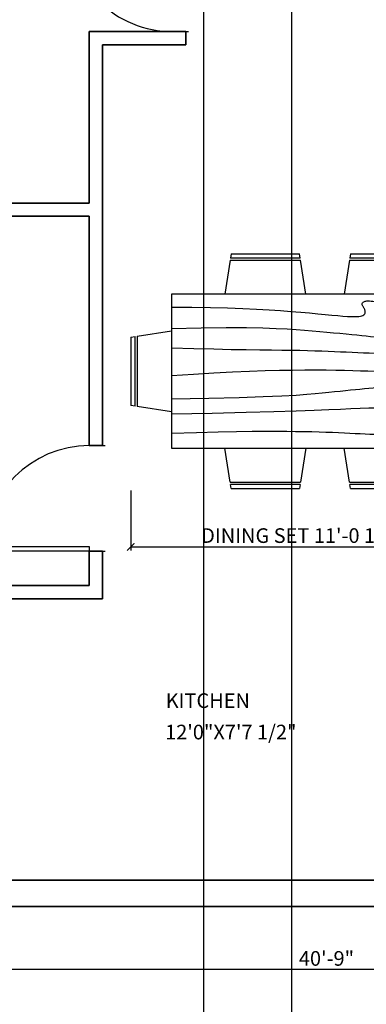
# Model space of a CAD drawing. Units: inches. Extents: x 3283068 to 3284536, y 3240756 to 3241803.
# Tile 6 of 19: x 3283479 to 3283598, y 3241165 to 3241501. Entities that reach past the tile are written whole.
import ezdxf

# ---------------------------------------------------------------- set-up
doc = ezdxf.new("R2010")
doc.units = ezdxf.units.IN
for name, color, linetype, lineweight in [('A-ANNO-DIMS', 2, 'Continuous', 18), ('A-AREA-IDEN', 7, 'Continuous', 18), ('door', 140, 'Continuous', 25), ('furniture', 40, 'Continuous', 18), ('wall', 20, 'Continuous', 35)]:
    doc.layers.add(name, color=color, linetype=linetype, lineweight=lineweight)
doc.layers.add('HATCH', color=8, linetype='Continuous')
doc.layers.add('NOI THAT', color=42, linetype='Continuous')
doc.styles.get("Standard").update_dxf_attribs({"font": 'arial.ttf'})
doc.dimstyles.new('ISO-25', dxfattribs={"dimtxt": 5, "dimasz": 2.5, "dimexe": 1.25, "dimexo": 0.625, "dimtad": 1, "dimlunit": 4, "dimtxsty": 'Standard', "dimblk": 'ARCHTICK', "dimcen": 2.5, "dimadec": 0, "dimazin": 0, "dimtfac": 1, "dimtmove": 0, "dimatfit": 3, "dimfxl": 1, "dimarcsym": 0})

# ---------------------------------------------------------------- blocks, each defined once
blk = doc.blocks.new('*U7')
for p, q in [((0, 0), (0, 6)), ((40, 0), (40, 6))]:
    blk.add_line(p, q)
blk.add_lwpolyline([(0, 0), (0, -40), (1.75, -40), (1.75, 0)], close=True)
blk.add_arc((0, 0), 40, 270, 0)
blk = doc.blocks.new('*U5')
for p, q in [((-40, 0), (-40, 6)), ((0, 0), (0, 6))]:
    blk.add_line(p, q)
blk.add_lwpolyline([(0, 0), (0, -40), (-1.75, -40), (-1.75, 0)], close=True)
blk.add_arc((0, 0), 40, 180, 270)
blk = doc.blocks.new('A$C78170A85')
at = {"layer": 'HATCH'}
for points in [[(171.5, 767.4), (258.6, 767), (337.5, 765.8), (408.9, 764), (473.5, 761.7), (532, 759), (585.1, 755.9), (633.5, 752.7), (677.8, 749.3), (718.8, 745.9), (756.5, 742.6), (790.9, 739.5), (822.2, 736.5), (850.3, 733.8), (875.4, 731.5), (897.3, 729.6), (916.3, 728.2), (932.4, 727.4), (945.8, 727.1), (956.7, 727.2), (965.6, 727.9), (972.6, 728.9), (978.1, 730.4), (982.3, 732.1), (985.5, 734.3), (988, 736.6), (989.8, 739.3), (991.1, 742.1), (991.7, 745), (991.9, 748), (991.7, 751), (991, 753.9), (990, 756.8), (988.8, 759.6), (987.3, 762.2), (985.8, 764.7), (984.2, 767.2), (982.7, 769.5), (981.4, 771.9), (980.3, 774.1), (979.5, 776.4), (979.2, 778.6), (979.2, 780.9), (979.7, 783), (980.6, 785), (982, 786.9), (983.7, 788.7), (985.9, 790.2), (988.5, 791.4), (991.6, 792.4), (995.2, 793.1), (999.4, 793.6), (1004.3, 793.7), (1010.1, 793.6), (1016.9, 793.1), (1024.7, 792.4), (1033.7, 791.4), (1043.9, 790.2), (1055.7, 788.6), (1069.2, 786.9), (1084.6, 784.9), (1102.1, 782.6), (1122, 780.2), (1144.5, 777.6), (1169.9, 774.9), (1198.1, 772), (1229.4, 769), (1263.4, 765.9), (1300.1, 762.7), (1339.4, 759.4), (1381.1, 756.1), (1425.2, 752.7), (1471.5, 749.3)], [(171.5, 677.1), (298.3, 679.7), (403.1, 680.8), (488.9, 680.7), (558.5, 679.5), (615, 677.6), (661.2, 675.2), (700.3, 672.4), (735, 669.6), (767.9, 666.8), (799.4, 664.2), (829.5, 661.7), (858.1, 659.2), (885.2, 656.9), (910.7, 654.5), (934.7, 652.3), (956.9, 650), (977.5, 647.8), (996.5, 645.6), (1013.9, 643.5), (1029.7, 641.5), (1044.1, 639.8), (1057, 638.4), (1068.6, 637.2), (1078.8, 636.5), (1087.8, 636.1), (1095.6, 636.2), (1102.4, 636.6), (1108.2, 637.4), (1113.1, 638.6), (1117.3, 640.1), (1120.9, 641.9), (1124, 644), (1126.6, 646.4), (1128.7, 649), (1130.4, 651.9), (1131.7, 654.9), (1132.4, 658.1), (1132.6, 661.3), (1132.3, 664.7), (1131.5, 668.1), (1130.1, 671.4), (1128.2, 674.8), (1126, 678.2), (1123.6, 681.6), (1121, 685), (1118.4, 688.4), (1115.8, 691.8), (1113.4, 695.1), (1111.3, 698.5), (1109.5, 701.9), (1108.2, 705.2), (1107.2, 708.5), (1106.8, 711.7), (1106.9, 714.8), (1107.6, 717.8), (1108.9, 720.7), (1110.9, 723.5), (1113.6, 726), (1116.9, 728.2), (1120.8, 730.1), (1125.1, 731.6), (1129.9, 732.6), (1135, 733), (1140.5, 732.8), (1146.3, 731.8), (1152.7, 730.3), (1159.9, 728.2), (1168.1, 725.5), (1177.6, 722.4), (1188.6, 718.9), (1201.5, 715.1), (1216.5, 710.9), (1233.8, 706.6), (1254.1, 701.9), (1277.9, 696.7), (1305.9, 690.9), (1338.7, 684.4), (1376.8, 677), (1420.9, 668.6), (1471.5, 659)], [(171.5, 595.8), (266.9, 592.9), (350.8, 590.6), (424.4, 588.9), (488.8, 587.7), (545.3, 586.9), (594.9, 586.3), (639, 585.8), (678.6, 585.3), (714.8, 584.7), (748.2, 583.9), (779.2, 583.1), (808.2, 582.1), (835.5, 581.1), (861.6, 580), (886.9, 578.9), (911.8, 577.8), (936.6, 576.7), (961.2, 575.6), (985.3, 574.6), (1008.9, 573.6), (1031.5, 572.9), (1053.1, 572.3), (1073.5, 571.9), (1092.4, 571.8), (1109.6, 571.9), (1125.2, 572.3), (1139.3, 573), (1152, 574), (1163.3, 575.3), (1173.4, 576.8), (1182.3, 578.7), (1190.2, 580.8), (1197, 583.2), (1203, 585.8), (1208.4, 588.6), (1213.1, 591.5), (1217.4, 594.5), (1221.5, 597.5), (1225.4, 600.5), (1229.3, 603.4), (1233.3, 606.1), (1237.5, 608.7), (1242, 611), (1246.8, 613.1), (1251.9, 615), (1257.4, 616.5), (1263.4, 617.6), (1269.9, 618.4), (1277, 618.8), (1284.5, 618.7), (1292.5, 618.3), (1300.9, 617.5), (1309.7, 616.3), (1318.8, 614.8), (1328.1, 613), (1337.6, 610.9), (1347.4, 608.5), (1357.9, 605.7), (1369.8, 602.5), (1383.7, 598.8), (1400.2, 594.6), (1419.9, 589.7), (1443.5, 584.1), (1471.5, 577.8)], [(171.5, 478.5), (265.6, 484.6), (351.7, 489.6), (430.6, 493.6), (502.7, 496.6), (568.7, 498.8), (629.2, 500.4), (684.7, 501.3), (735.8, 501.8), (783, 501.9), (826.7, 501.7), (867.2, 501.3), (904.8, 500.6), (939.8, 499.7), (972.5, 498.7), (1003.2, 497.6), (1032.2, 496.5), (1059.7, 495.4), (1085.8, 494.3), (1110.4, 493.4), (1133.6, 492.6), (1155.2, 492), (1175.4, 491.7), (1194.1, 491.7), (1211.2, 492), (1226.8, 492.8), (1241.1, 493.9), (1254, 495.3), (1266, 496.9), (1277, 498.7), (1287.2, 500.5), (1296.8, 502.3), (1306, 504.1), (1314.9, 505.7), (1323.7, 507.1), (1332.3, 508.3), (1341, 509.3), (1349.8, 510), (1358.9, 510.4), (1368.3, 510.4), (1378.2, 510.1), (1388.6, 509.3), (1399.3, 508.2), (1409.9, 506.9), (1420.3, 505.4), (1430, 503.8), (1438.9, 502.2), (1446.5, 500.8), (1452.7, 499.5), (1457.3, 498.5), (1460.4, 497.8), (1462.6, 497.3), (1464.1, 496.9), (1465.4, 496.7), (1466.8, 496.6), (1468.7, 496.5), (1471.5, 496.5)], [(171.5, 379.2), (330.7, 382.5), (458.9, 385.9), (560.3, 389.2), (639, 392.5), (699.2, 395.7), (745, 398.8), (780.7, 401.9), (810.2, 404.7), (837.3, 407.5), (862.5, 410.1), (886.3, 412.6), (908.7, 414.9), (929.9, 417.1), (950.2, 419.1), (969.7, 421), (988.5, 422.8), (1007, 424.4), (1025.1, 425.9), (1043, 427.1), (1060.8, 428.1), (1078.6, 428.8), (1096.5, 429.1), (1114.6, 429.2), (1133, 428.8), (1151.8, 428.1), (1170.8, 426.9), (1189.9, 425.5), (1208.8, 423.7), (1227.3, 421.8), (1245.3, 419.7), (1262.6, 417.5), (1278.9, 415.3), (1294.2, 413), (1308.5, 410.8), (1321.9, 408.5), (1334.7, 406.3), (1346.9, 404.2), (1358.8, 402.1), (1370.4, 400), (1382, 398), (1393.6, 396.1), (1405.2, 394.4), (1416.7, 393), (1428.2, 392.2), (1439.4, 392.1), (1450.5, 392.8), (1461.2, 394.4), (1471.5, 397.2)], [(171.5, 316), (344.8, 319.3), (488.1, 322.7), (605.2, 325.9), (699.8, 328.9), (776, 331.8), (837.4, 334.4), (887.9, 336.6), (931.4, 338.5), (971, 340), (1007.5, 341.1), (1041.3, 341.9), (1072.4, 342.3), (1101.2, 342.5), (1127.7, 342.4), (1152.3, 342), (1175.1, 341.6), (1196.4, 340.9), (1216.4, 340.2), (1235.3, 339.3), (1253.5, 338.3), (1271.3, 337.2), (1288.7, 335.9), (1306.3, 334.6), (1324.1, 333.3), (1342.4, 331.8), (1361.1, 330.4), (1380, 329), (1398.9, 327.7), (1417.7, 326.6), (1436.2, 325.8), (1454.2, 325.2), (1471.5, 325)], [(171.5, 234.7), (278.3, 237.7), (369.5, 239.9), (447.2, 241.5), (513.2, 242.4), (569.3, 242.9), (617.5, 243), (659.5, 242.7), (697.4, 242.2), (732.7, 241.6), (765.7, 240.9), (796.8, 240), (825.9, 239), (853.4, 238), (879.3, 237), (903.7, 235.8), (926.9, 234.7), (948.9, 233.6), (970.2, 232.5), (991.1, 231.5), (1012, 230.7), (1033.1, 230), (1055, 229.5), (1077.9, 229.3), (1102.1, 229.5), (1128.4, 230), (1157.6, 231), (1191.3, 232.9), (1230.7, 235.8), (1277.1, 239.9), (1331.8, 245.4), (1396.2, 252.7), (1471.5, 261.8)]]:
    blk.add_lwpolyline(points, dxfattribs=at)
at = {"layer": 'NOI THAT'}
for p, q in [((420.1, 966), (397.5, 821.5)), ((420.1, 966), (717.5, 966)), ((424.3, 993.1), (421.5, 975)), ((716.1, 975), (421.5, 975)), ((424.3, 993.1), (713.2, 993.1)), ((716, 975), (713.2, 993.1)), ((740, 821.5), (717.4, 966)), ((925.6, 966), (903.1, 821.5)), ((925.7, 966), (1223.1, 966)), ((929.9, 993.1), (927, 975)), ((1221.6, 975), (927.1, 975)), ((929.9, 993.1), (1218.8, 993.1)), ((1221.6, 975), (1218.8, 993.1)), ((1245.6, 821.5), (1223, 966)), ((1471.5, 821.5), (171.5, 821.5)), ((171.5, 821.5), (171.5, 171.5)), ((1471.5, 171.5), (1471.5, 821.5)), ((27.1, 645.2), (171.6, 667.8)), ((1616, 645.2), (1471.5, 667.8)), ((0, 641), (18, 643.8)), ((0, 641), (0, 352.1)), ((18.1, 349.2), (18.1, 643.7)), ((27.1, 645.1), (27.1, 347.8)), ((1616, 645.1), (1616, 347.8)), ((1643.1, 641), (1625, 643.8)), ((1625, 349.2), (1625, 643.7)), ((1643.1, 641), (1643.1, 352.1)), ((18.1, 349.3), (0, 352.1)), ((171.6, 325.3), (27.1, 347.8)), ((1471.5, 325.3), (1616, 347.8)), ((1625, 349.3), (1643.1, 352.1)), ((420.1, 27.1), (397.5, 171.6)), ((740, 171.6), (717.4, 27.1)), ((925.6, 27.1), (903.1, 171.6)), ((1245.6, 171.6), (1223, 27.1)), ((420.1, 27.1), (717.5, 27.1)), ((716.1, 18.1), (421.5, 18.1)), ((424.3, 0), (421.5, 18)), ((424.3, 0), (713.2, 0)), ((716, 18.1), (713.2, 0)), ((925.7, 27.1), (1223.1, 27.1)), ((929.9, 0), (927, 18)), ((1221.6, 18.1), (927.1, 18.1)), ((929.9, 0), (1218.8, 0)), ((1221.6, 18.1), (1218.8, 0))]:
    blk.add_line(p, q, dxfattribs=at)
at = {"layer": 'NOI THAT', "ltscale": 20}
blk.add_line((171.5, 171.5), (1471.5, 171.5), dxfattribs=at)
blk = doc.blocks.new('_ArchTick')
at = {"color": 0, "linetype": 'ByBlock', "const_width": 0.15}
blk.add_lwpolyline([(-0.5, -0.5), (0.5, 0.5)], dxfattribs=at)
blk = doc.blocks.new('*D29')
at = {"layer": 'A-ANNO-DIMS', "color": 0, "lineweight": -2, "transparency": 16777216}
for p, q in [((3283339.59, 3241197.48), (3283339.59, 3241175.31)), ((3283828.59, 3241197.48), (3283828.59, 3241175.31)), ((3283828.59, 3241176.56), (3283339.59, 3241176.56))]:
    blk.add_line(p, q, dxfattribs=at)
at = {"layer": 'Defpoints', "color": 0, "transparency": 16777216}
for p in [(3283339.59, 3241198.1), (3283828.59, 3241198.1), (3283339.59, 3241176.56)]:
    blk.add_point(p, dxfattribs=at)
at = {"layer": 'A-ANNO-DIMS', "color": 0, "lineweight": -2, "transparency": 16777216, "xscale": 2.5, "yscale": 2.5, "zscale": 2.5, "rotation": 180}
blk.add_blockref('_ArchTick', (3283339.59, 3241176.56), dxfattribs=at)
at = {"layer": 'A-ANNO-DIMS', "color": 0, "lineweight": -2, "transparency": 16777216, "xscale": 2.5, "yscale": 2.5, "zscale": 2.5}
blk.add_blockref('_ArchTick', (3283828.59, 3241176.56), dxfattribs=at)
at = {"layer": 'A-ANNO-DIMS', "color": 0, "transparency": 16777216, "insert": (3283584.09, 3241179.74), "char_height": 5, "attachment_point": 5}
blk.add_mtext('40\'-9"', dxfattribs=at)
blk = doc.blocks.new('*D53')
at = {"layer": 'A-ANNO-DIMS', "color": 0, "lineweight": -2, "transparency": 16777216}
for p, q in [((3283517.27, 3241340.06), (3283517.27, 3241319.55)), ((3283649.87, 3241340.06), (3283649.87, 3241319.55)), ((3283517.27, 3241320.8), (3283649.87, 3241320.8))]:
    blk.add_line(p, q, dxfattribs=at)
at = {"layer": 'Defpoints', "color": 0, "transparency": 16777216}
for p in [(3283517.27, 3241340.69), (3283649.87, 3241340.69), (3283649.87, 3241320.8)]:
    blk.add_point(p, dxfattribs=at)
at = {"layer": 'A-ANNO-DIMS', "color": 0, "lineweight": -2, "transparency": 16777216, "xscale": 2.5, "yscale": 2.5, "zscale": 2.5, "rotation": 180}
blk.add_blockref('_ArchTick', (3283517.27, 3241320.8), dxfattribs=at)
at = {"layer": 'A-ANNO-DIMS', "color": 0, "lineweight": -2, "transparency": 16777216, "xscale": 2.5, "yscale": 2.5, "zscale": 2.5}
blk.add_blockref('_ArchTick', (3283649.87, 3241320.8), dxfattribs=at)
at = {"layer": 'A-ANNO-DIMS', "color": 0, "transparency": 16777216, "insert": (3283583.57, 3241324.01), "char_height": 5, "attachment_point": 5}
blk.add_mtext('DINING SET 11\'-0 1/2" TYP.', dxfattribs=at)
blk = doc.blocks.new('*D63')
at = {"layer": 'A-ANNO-DIMS', "color": 0, "lineweight": -2, "transparency": 16777216}
for p, q in [((3283248.09, 3241083.23), (3283248.09, 3241798.08)), ((3283248.09, 3241796.83), (3284328.09, 3241796.83)), ((3284328.09, 3241083.23), (3284328.09, 3241798.08))]:
    blk.add_line(p, q, dxfattribs=at)
at = {"layer": 'Defpoints', "color": 0, "transparency": 16777216}
for p in [(3284328.09, 3241796.83), (3283248.09, 3241082.6), (3284328.09, 3241082.6)]:
    blk.add_point(p, dxfattribs=at)
at = {"layer": 'A-ANNO-DIMS', "color": 0, "lineweight": -2, "transparency": 16777216, "xscale": 2.5, "yscale": 2.5, "zscale": 2.5, "rotation": 180}
blk.add_blockref('_ArchTick', (3283248.09, 3241796.83), dxfattribs=at)
at = {"layer": 'A-ANNO-DIMS', "color": 0, "lineweight": -2, "transparency": 16777216, "xscale": 2.5, "yscale": 2.5, "zscale": 2.5}
blk.add_blockref('_ArchTick', (3284328.09, 3241796.83), dxfattribs=at)
at = {"layer": 'A-ANNO-DIMS', "color": 0, "transparency": 16777216, "insert": (3283788.09, 3241800.01), "char_height": 5, "attachment_point": 5}
blk.add_mtext('90\'-0"', dxfattribs=at)
blk = doc.blocks.new('*D64')
at = {"layer": 'A-ANNO-DIMS', "color": 0, "lineweight": -2, "transparency": 16777216}
for p, q in [((3283542.09, 3241534.98), (3283542.09, 3240759.03)), ((3283572.09, 3241534.98), (3283572.09, 3240759.03)), ((3283542.09, 3240760.28), (3283572.09, 3240760.28))]:
    blk.add_line(p, q, dxfattribs=at)
at = {"layer": 'Defpoints', "color": 0, "transparency": 16777216}
for p in [(3283542.09, 3241535.6), (3283572.09, 3241535.6), (3283572.09, 3240760.28)]:
    blk.add_point(p, dxfattribs=at)
at = {"layer": 'A-ANNO-DIMS', "color": 0, "lineweight": -2, "transparency": 16777216, "xscale": 2.5, "yscale": 2.5, "zscale": 2.5, "rotation": 180}
blk.add_blockref('_ArchTick', (3283542.09, 3240760.28), dxfattribs=at)
at = {"layer": 'A-ANNO-DIMS', "color": 0, "lineweight": -2, "transparency": 16777216, "xscale": 2.5, "yscale": 2.5, "zscale": 2.5}
blk.add_blockref('_ArchTick', (3283572.09, 3240760.28), dxfattribs=at)
at = {"layer": 'A-ANNO-DIMS', "color": 0, "transparency": 16777216, "insert": (3283557.09, 3240763.46), "char_height": 5, "attachment_point": 5}
blk.add_mtext('2\'-6"', dxfattribs=at)

msp = doc.modelspace()

# ---------------------------------------------------------------- linework, layer by layer
at = {"layer": 'door'}
for p, q in [((3283507.589, 3241355.345), (3283503.089, 3241355.345)), ((3283507.589, 3241319.345), (3283503.089, 3241319.345))]:
    msp.add_line(p, q, dxfattribs=at)
at = {"layer": 'wall'}
for p, q in [((3283503.089, 3241496.602), (3283536.089, 3241496.602)), ((3283503.089, 3241496.602), (3283531.589, 3241496.602)), ((3283503.089, 3241496.602), (3283503.089, 3241438.102)), ((3283536.089, 3241496.602), (3283536.089, 3241492.102)), ((3283507.589, 3241492.102), (3283507.589, 3241355.345)), ((3283507.589, 3241492.102), (3283536.089, 3241492.102)), ((3283507.589, 3241492.102), (3283531.589, 3241492.102)), ((3283348.589, 3241438.102), (3283503.089, 3241438.102)), ((3283348.589, 3241433.602), (3283503.089, 3241433.602)), ((3283503.089, 3241433.602), (3283503.089, 3241355.345)), ((3283503.089, 3241319.345), (3283503.089, 3241307.602)), ((3283507.589, 3241319.345), (3283507.589, 3241303.102)), ((3283348.589, 3241307.602), (3283503.089, 3241307.602)), ((3283461.089, 3241303.102), (3283507.589, 3241303.102)), ((3283461.089, 3241207.102), (3283605.089, 3241207.102)), ((3283339.589, 3241198.102), (3284236.589, 3241198.102))]:
    msp.add_line(p, q, dxfattribs=at)

# ---------------------------------------------------------------- block references
at = {"layer": 'door', "xscale": 0.9, "yscale": 0.9, "zscale": 0.9, "rotation": 270}
for name, p in [('*U7', (3283531.589, 3241532.602)), ('*U5', (3283503.089, 3241319.345))]:
    msp.add_blockref(name, p, dxfattribs=at)
at = {"layer": 'furniture', "xscale": 0.0807042311318891, "yscale": 0.0807042311318891, "zscale": 0.0807042311318891}
msp.add_blockref('A$C78170A85', (3283517.269, 3241340.686), dxfattribs=at)

# ---------------------------------------------------------------- texts
at = {"layer": 'A-AREA-IDEN'}
for s, p in [('KITCHEN', (3283529.187, 3241265.847)), ('12\'0"X7\'7 1/2"', (3283528.984, 3241255.124))]:
    msp.add_text(s, height=5, dxfattribs=at).set_placement(p)

# ---------------------------------------------------------------- dimensions: what is measured, and where the dimension line sits
at = {"layer": 'A-ANNO-DIMS'}
for base, p1, p2, override, picture, middle in [((3284328.089, 3241796.827), (3283248.089, 3241082.602), (3284328.089, 3241082.602), {"dimdec": 1, "dimlfac": 1, "dimrnd": 0, "dimzin": 1, "dimdsep": 46, "dimlunit": 4, "dimfrac": 2}, '*D63', (3283788.089, 3241800.005)), ((3283572.089, 3240760.281), (3283542.089, 3241535.602), (3283572.089, 3241535.602), {"dimdec": 1, "dimlfac": 1, "dimrnd": 0, "dimzin": 1, "dimdsep": 46, "dimlunit": 4, "dimfrac": 2}, '*D64', (3283557.089, 3240763.459)), ((3283339.589, 3241176.561), (3283828.589, 3241198.102), (3283339.589, 3241198.102), {"dimclrd": 0, "dimclre": 0, "dimclrt": 0}, '*D29', (3283584.089, 3241179.739))]:
    dim = msp.add_linear_dim(base=base, p1=p1, p2=p2, dimstyle='ISO-25', override=override, dxfattribs=at)
    dim.commit()
    dim.dimension.update_dxf_attribs({"geometry": picture, "text_midpoint": middle})
dim = msp.add_linear_dim(base=(3283649.87, 3241320.796), p1=(3283517.269, 3241340.686), p2=(3283649.87, 3241340.686), text='DINING SET <> TYP.', dimstyle='ISO-25', override={"dimdec": 1, "dimlfac": 1, "dimrnd": 0, "dimzin": 1, "dimdsep": 46, "dimlunit": 4, "dimfrac": 2}, dxfattribs=at)
dim.commit()
dim.dimension.update_dxf_attribs({"geometry": '*D53', "text_midpoint": (3283583.57, 3241324.006)})

doc.saveas('drawing.dxf')
